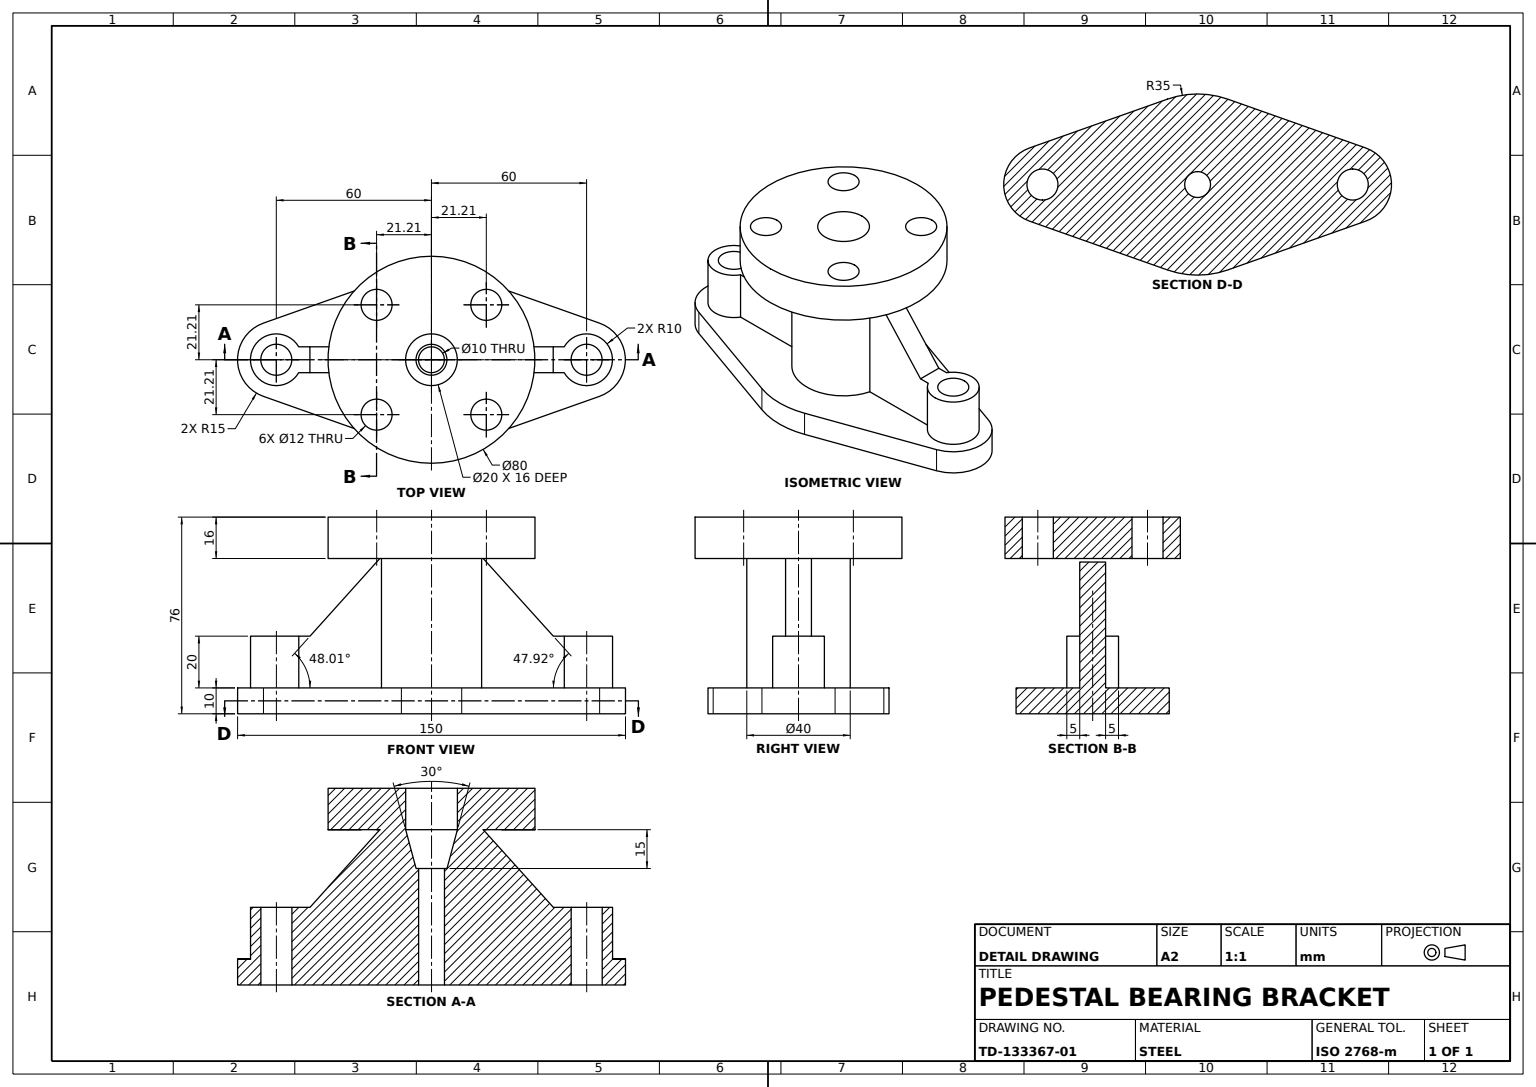
from build123d import *

# Parameters (mm, degrees)
BASE_FLANGE_SKETCH_R                 = 5
BASE_FLANGE_SKETCH_R_2               = 6
BASE_FLANGE_DEPTH                    = 10
PILLAR_AND_LUG_BOSSES_SKETCH_R       = 20
PILLAR_AND_LUG_BOSSES_SKETCH_R_2     = 5
PILLAR_AND_LUG_BOSSES_SKETCH_R_3     = 10
PILLAR_AND_LUG_BOSSES_SKETCH_R_4     = 6
PILLAR_AND_LUG_BOSSES_DEPTH          = 20
UPPER_PILLAR_SKETCH_R                = 20
UPPER_PILLAR_SKETCH_R_2              = 5
UPPER_PILLAR_40_DEPTH                = 30
SUPPORT_WEB_DEPTH                    = 5
TAPERED_BORE_SKETCH_R                = 10
TAPERED_BORE_20_DEPTH                = 15
TAPERED_BORE_20_DRAFT                = -15
TOP_FLANGE_SKETCH_R                  = 40
TOP_FLANGE_SKETCH_R_2                = 10
TOP_FLANGE_SKETCH_R_3                = 6
TOP_FLANGE_80_WITH_HOLES_4X_12_DEPTH = 16


with BuildPart() as part:
    # Base Flange Sketch → Base Flange (new body)
    with BuildSketch(Plane(origin=(0, 0, 0), x_dir=(1, 0, 0), z_dir=(0, 1, 0))):
        with BuildLine():
            Line((-11.666666667, 32.998316455), (-65, 14.142135624))
            ThreePointArc((-65, 14.142135624), (-75, 0), (-65, -14.142135624))
            Line((-65, -14.142135624), (-11.666666667, -32.998316455))
            ThreePointArc((-11.666666667, -32.998316455), (0, -35), (11.666666667, -32.998316455))
            Line((11.666666667, -32.998316455), (65, -14.142135624))
            ThreePointArc((65, -14.142135624), (75, 0), (65, 14.142135624))
            Line((65, 14.142135624), (11.666666667, 32.998316455))
            ThreePointArc((11.666666667, 32.998316455), (0, 35), (-11.666666667, 32.998316455))
        make_face()
        with Locations(Location((0, 0, 0), (0, 0, 270))):
            Circle(BASE_FLANGE_SKETCH_R, mode=Mode.SUBTRACT)
        with Locations(Location((-60, 0, 0), (0, 0, 270))):
            Circle(BASE_FLANGE_SKETCH_R_2, mode=Mode.SUBTRACT)
        with Locations(Location((60, 0, 0), (0, 0, 270))):
            Circle(BASE_FLANGE_SKETCH_R_2, mode=Mode.SUBTRACT)
    extrude(amount=BASE_FLANGE_DEPTH)

    # Pillar and Lug Bosses Sketch → Pillar and Lug Bosses (add)
    # profile 1 of 3: a face of its own
    with BuildSketch(Plane(origin=(0, 10, 0), x_dir=(1, 0, 0), z_dir=(0, 1, 0))):
        with Locations(Location((0, 0, 0), (0, 0, 270))):
            Circle(PILLAR_AND_LUG_BOSSES_SKETCH_R)
        with Locations(Location((0, 0, 0), (0, 0, 270))):
            Circle(PILLAR_AND_LUG_BOSSES_SKETCH_R_2, mode=Mode.SUBTRACT)
    # profile 2 of 3: a face of its own
    with BuildSketch(Plane(origin=(0, 10, 0), x_dir=(1, 0, 0), z_dir=(0, 1, 0))):
        with Locations(Location((-60, 0, 0), (0, 0, 270))):
            Circle(PILLAR_AND_LUG_BOSSES_SKETCH_R_3)
        with Locations(Location((-60, 0, 0), (0, 0, 270))):
            Circle(PILLAR_AND_LUG_BOSSES_SKETCH_R_4, mode=Mode.SUBTRACT)
    # profile 3 of 3: a face of its own
    with BuildSketch(Plane(origin=(0, 10, 0), x_dir=(1, 0, 0), z_dir=(0, 1, 0))):
        with Locations(Location((60, 0, 0), (0, 0, 270))):
            Circle(PILLAR_AND_LUG_BOSSES_SKETCH_R_3)
        with Locations(Location((60, 0, 0), (0, 0, 270))):
            Circle(PILLAR_AND_LUG_BOSSES_SKETCH_R_4, mode=Mode.SUBTRACT)
    extrude(amount=PILLAR_AND_LUG_BOSSES_DEPTH)

    # Upper Pillar Sketch → Upper Pillar Ø40 (add)
    with BuildSketch(Plane(origin=(0, 30, 0), x_dir=(1, 0, 0), z_dir=(0, 1, 0))):
        with Locations(Location((0, 0, 0), (0, 0, 270))):
            Circle(UPPER_PILLAR_SKETCH_R)
        with Locations(Location((0, 0, 0), (0, 0, 270))):
            Circle(UPPER_PILLAR_SKETCH_R_2, mode=Mode.SUBTRACT)
    extrude(amount=UPPER_PILLAR_40_DEPTH)

    # Support Web Sketch → Support Web (add, symmetric)
    with BuildSketch(Plane.XY):
        Polygon((-47, 30), (-52, 30), (-52, 10), (-16.568658107, 10), (-16.568658107, 60), (-20, 60), align=None)
        Polygon((52.090777917, 30), (47.090777917, 30), (20, 60), (17.352207011, 60), (17.352207011, 10), (52.090777917, 10), align=None)
    extrude(amount=SUPPORT_WEB_DEPTH, both=True)


with BuildPart() as tapered_bore_20_tool:
    # Tapered Bore Sketch → Tapered Bore Ø20 (with draft: the straight prism first)
    with BuildSketch(Plane(origin=(0, 60, 0), x_dir=(1, 0, 0), z_dir=(0, 1, 0))):
        Circle(TAPERED_BORE_SKETCH_R)
    extrude(amount=-TAPERED_BORE_20_DEPTH)
    # Tapered Bore Ø20: the draft: its side faces are tilted about the plane it starts from
    tapered_bore_20_sides = [tapered_bore_20_tool.faces().sort_by_distance(p)[0] for p in [
        (-10, 52.5, 0),
    ]]
    draft(tapered_bore_20_sides, Plane(origin=(0, 60, 0), x_dir=(1, 0, 0), z_dir=(0, 1, 0)), TAPERED_BORE_20_DRAFT)


with BuildPart() as part_1:
    add(part.part)

    # Tapered Bore Ø20: cut by tapered_bore_20_tool
    add(tapered_bore_20_tool.part, mode=Mode.SUBTRACT)

    # Top Flange Sketch → Top Flange Ø80 with Holes 4xØ12 (add)
    with BuildSketch(Plane(origin=(0, 60, 0), x_dir=(1, 0, 0), z_dir=(0, 1, 0))):
        with Locations(Location((0, 0, 0), (0, 0, 270))):
            Circle(TOP_FLANGE_SKETCH_R)
        with Locations(Location((0, 0, 0), (0, 0, 270))):
            Circle(TOP_FLANGE_SKETCH_R_2, mode=Mode.SUBTRACT)
        with Locations(Location((21.213203436, 21.213203436, 0), (0, 0, 270))):
            Circle(TOP_FLANGE_SKETCH_R_3, mode=Mode.SUBTRACT)
        with Locations(Location((21.213203436, -21.213203436, 0), (0, 0, 270))):
            Circle(TOP_FLANGE_SKETCH_R_3, mode=Mode.SUBTRACT)
        with Locations(Location((-21.213203436, -21.213203436, 0), (0, 0, 270))):
            Circle(TOP_FLANGE_SKETCH_R_3, mode=Mode.SUBTRACT)
        with Locations(Location((-21.213203436, 21.213203436, 0), (0, 0, 270))):
            Circle(TOP_FLANGE_SKETCH_R_3, mode=Mode.SUBTRACT)
    extrude(amount=TOP_FLANGE_80_WITH_HOLES_4X_12_DEPTH)


solid = part_1.part
